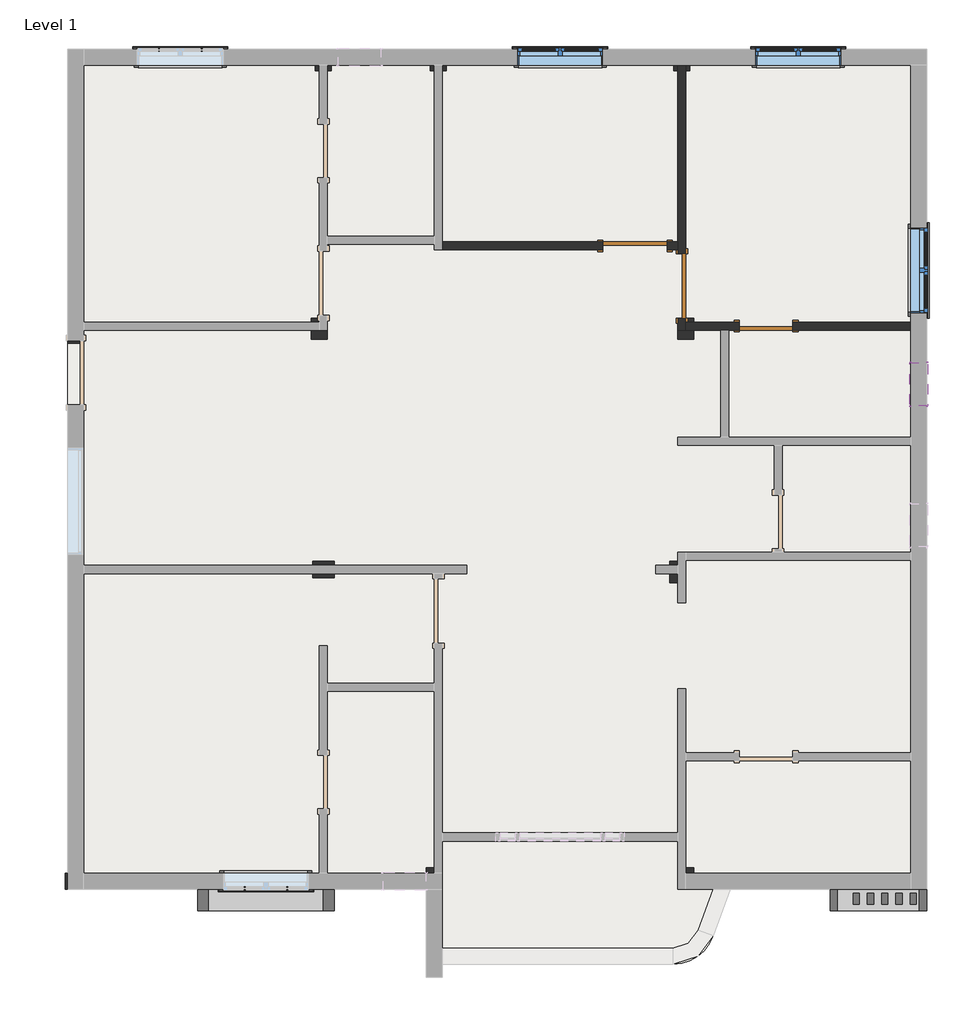
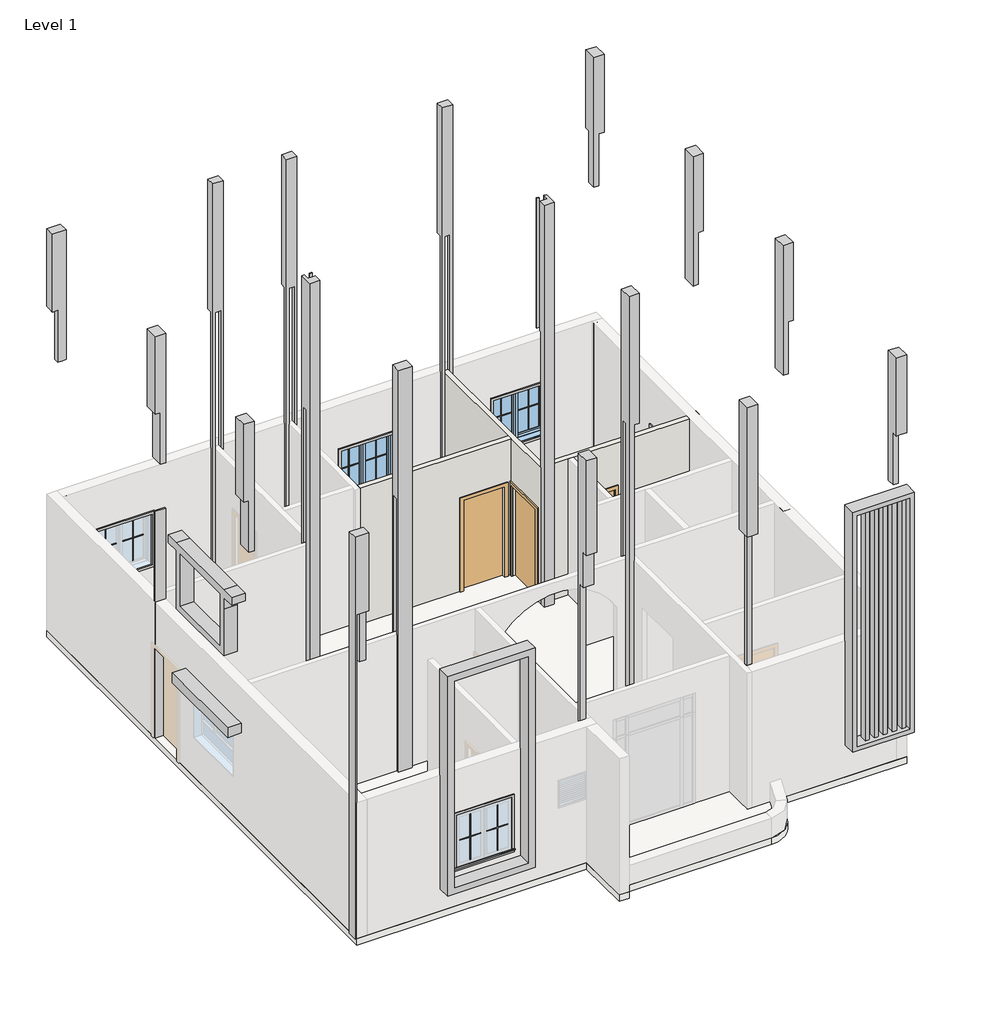
# One storey, part 2 of 2: 21 proxies, 17 columns, 4 windows, 3 doors, 3 walls, 1 slab.
# Revit data of these elements (continued)
# Element 48 (IfcWindow, "Window-Casement-Double : 48\" x 48\"") (continued)
#   Exterior Trim Visibility = yes
#   Phase Created = New Construction
#   Materials on its faces: "Wood - Stained", "Glass", "Clad - White"
# Element 49 (IfcWindow, "Window-Louvers : 24\" x 24\"")
#   Mark = "3"
#   Blade Width = 1' - 10 1/2"
#   Phase Created = New Construction
#   Materials on its faces: "Birch"
# Materials
#   "Door - Panel": class "Wood", colour RGB 210 159 95, transparency 0, Cost = 0
#   "Door - Frame": colour RGB 118 70 51, transparency 0, Cost = 0
#   "Gypsum Wall Board": class "Generic", colour RGB 127 127 127, transparency 0, Description = "Gypsum Wall Board", Cost = 0
#   "Wood - Stained": class "Wood", colour RGB 224 178 126, transparency 0, Cost = 0
#   "Glass": class "Glass", colour RGB 0 128 192, transparency 0.75, Description = "Soda Lime Glass", Cost = 0
#   "Clad - White": class "Wood", colour RGB 242 242 238, transparency 0, Cost = 0
#   "Birch": class "Wood", colour RGB 224 178 126, transparency 0, Description = "Betula Alleghaniensis", Cost = 0
#   "EIFS, Exterior Insulation": class "Generic", colour RGB 127 127 127, transparency 0, Description = "EIFS - Exterior Insulation", Cost = 0
#   "Brick, Common": class "Masonry", colour RGB 170 98 104, transparency 0, Description = "Common brick", Cost = 0
#   "Brick, Soldier Course": class "Masonry", colour RGB 170 98 104, transparency 0, Description = "Common brick soldier coursed", Cost = 0
#   "Electrical Analytical Loads": colour RGB 94 94 205, transparency 0.5, Cost = 0
